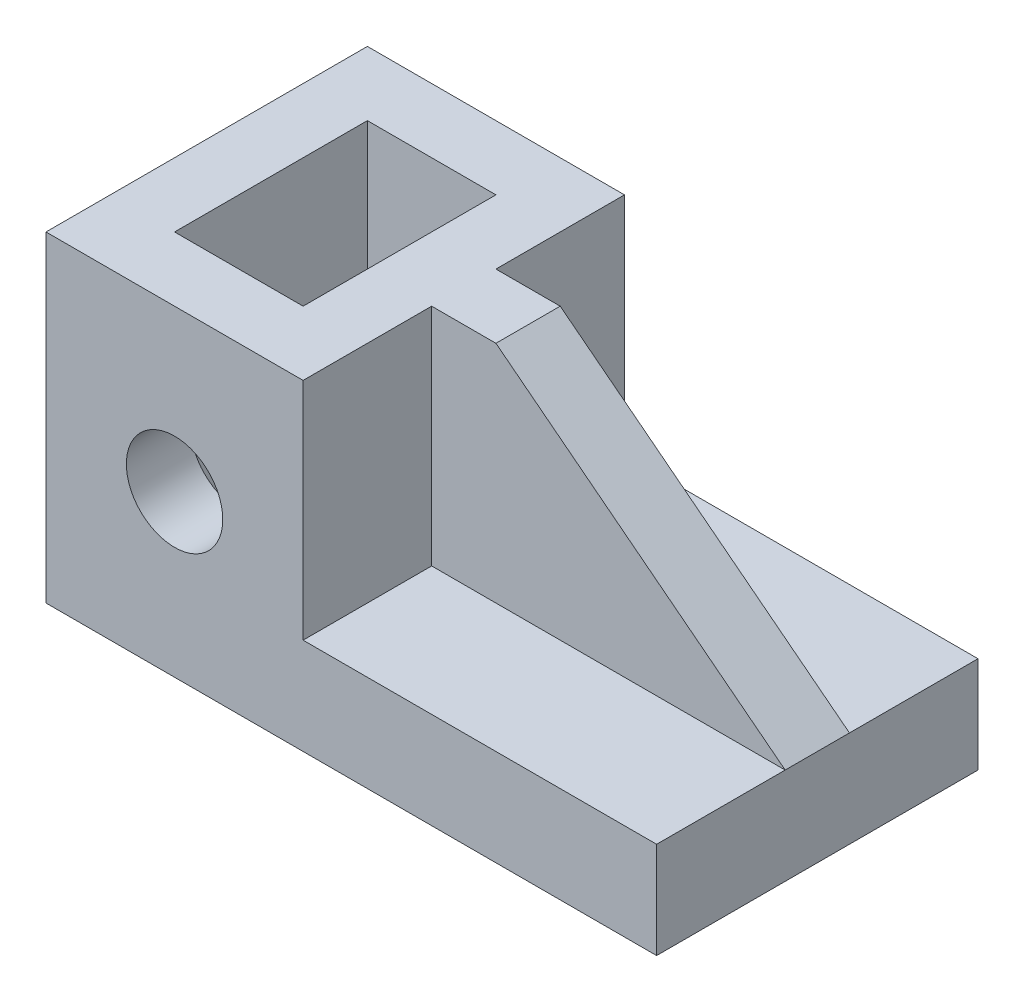
ISO-10303-21;
HEADER;
FILE_DESCRIPTION(('STEP AP214'),'2;1');
FILE_NAME('part.step','',(''),(''),'','','');
FILE_SCHEMA(('AUTOMOTIVE_DESIGN { 1 0 10303 214 1 1 1 1 }'));
ENDSEC;
DATA;
#1=APPLICATION_CONTEXT('core data for automotive mechanical design processes');
#2=APPLICATION_PROTOCOL_DEFINITION('international standard','automotive_design',2000,#1);
#3=PRODUCT_CONTEXT('',#1,'mechanical');
#4=PRODUCT('Part','Part','',(#3));
#5=PRODUCT_RELATED_PRODUCT_CATEGORY('part','',(#4));
#6=PRODUCT_DEFINITION_FORMATION('','',#4);
#7=PRODUCT_DEFINITION_CONTEXT('part definition',#1,'design');
#8=PRODUCT_DEFINITION('design','',#6,#7);
#9=PRODUCT_DEFINITION_SHAPE('','',#8);
#10=(LENGTH_UNIT() NAMED_UNIT(*) SI_UNIT(.MILLI.,.METRE.));
#11=(NAMED_UNIT(*) PLANE_ANGLE_UNIT() SI_UNIT($,.RADIAN.));
#12=(NAMED_UNIT(*) SI_UNIT($,.STERADIAN.) SOLID_ANGLE_UNIT());
#13=UNCERTAINTY_MEASURE_WITH_UNIT(LENGTH_MEASURE(1.E-05),#10,'distance_accuracy_value','');
#14=(GEOMETRIC_REPRESENTATION_CONTEXT(3) GLOBAL_UNCERTAINTY_ASSIGNED_CONTEXT((#13)) GLOBAL_UNIT_ASSIGNED_CONTEXT((#10,
#11,#12)) REPRESENTATION_CONTEXT('',''));
#15=CARTESIAN_POINT('',(0.,0.,0.));
#16=DIRECTION('',(0.,0.,1.));
#17=DIRECTION('',(1.,0.,0.));
#18=AXIS2_PLACEMENT_3D('',#15,#16,#17);
#19=CARTESIAN_POINT('',(40.,15.,50.));
#20=DIRECTION('',(0.,-1.,0.));
#21=DIRECTION('',(0.,0.,-1.));
#22=AXIS2_PLACEMENT_3D('',#19,#20,#21);
#23=PLANE('',#22);
#24=DIRECTION('',(-1.,0.,0.));
#25=VECTOR('',#24,1.);
#26=CARTESIAN_POINT('',(50.,15.,20.));
#27=LINE('',#26,#25);
#28=CARTESIAN_POINT('',(95.,15.,20.));
#29=VERTEX_POINT('',#28);
#30=CARTESIAN_POINT('',(40.,15.,20.));
#31=VERTEX_POINT('',#30);
#32=EDGE_CURVE('E189',#29,#31,#27,.T.);
#33=ORIENTED_EDGE('',*,*,#32,.F.);
#34=DIRECTION('',(0.,0.,-1.));
#35=VECTOR('',#34,1.);
#36=CARTESIAN_POINT('',(95.,15.,50.));
#37=LINE('',#36,#35);
#38=CARTESIAN_POINT('',(95.,15.,0.));
#39=VERTEX_POINT('',#38);
#40=EDGE_CURVE('E254',#29,#39,#37,.T.);
#41=ORIENTED_EDGE('',*,*,#40,.T.);
#42=DIRECTION('',(-1.,0.,0.));
#43=VECTOR('',#42,1.);
#44=CARTESIAN_POINT('',(40.,15.,0.));
#45=LINE('',#44,#43);
#46=CARTESIAN_POINT('',(40.,15.,0.));
#47=VERTEX_POINT('',#46);
#48=EDGE_CURVE('E236',#39,#47,#45,.T.);
#49=ORIENTED_EDGE('',*,*,#48,.T.);
#50=DIRECTION('',(0.,0.,-1.));
#51=VECTOR('',#50,1.);
#52=CARTESIAN_POINT('',(40.,15.,50.));
#53=LINE('',#52,#51);
#54=EDGE_CURVE('E253',#31,#47,#53,.T.);
#55=ORIENTED_EDGE('',*,*,#54,.F.);
#56=EDGE_LOOP('',(#33,#41,#49,#55));
#57=FACE_BOUND('',#56,.T.);
#58=ADVANCED_FACE('F39',(#57),#23,.F.);
#59=CARTESIAN_POINT('',(40.,50.,50.));
#60=DIRECTION('',(-1.,0.,0.));
#61=DIRECTION('',(0.,0.,1.));
#62=AXIS2_PLACEMENT_3D('',#59,#60,#61);
#63=PLANE('',#62);
#64=DIRECTION('',(0.,0.,-1.));
#65=VECTOR('',#64,1.);
#66=CARTESIAN_POINT('',(40.,50.,50.));
#67=LINE('',#66,#65);
#68=CARTESIAN_POINT('',(40.,50.,20.));
#69=VERTEX_POINT('',#68);
#70=CARTESIAN_POINT('',(40.,50.,0.));
#71=VERTEX_POINT('',#70);
#72=EDGE_CURVE('E250',#69,#71,#67,.T.);
#73=ORIENTED_EDGE('',*,*,#72,.F.);
#74=DIRECTION('',(0.,1.,0.));
#75=VECTOR('',#74,1.);
#76=CARTESIAN_POINT('',(40.,15.,20.));
#77=LINE('',#76,#75);
#78=EDGE_CURVE('E200',#31,#69,#77,.T.);
#79=ORIENTED_EDGE('',*,*,#78,.F.);
#80=ORIENTED_EDGE('',*,*,#54,.T.);
#81=DIRECTION('',(0.,1.,0.));
#82=VECTOR('',#81,1.);
#83=CARTESIAN_POINT('',(40.,50.,0.));
#84=LINE('',#83,#82);
#85=EDGE_CURVE('E242',#47,#71,#84,.T.);
#86=ORIENTED_EDGE('',*,*,#85,.T.);
#87=EDGE_LOOP('',(#73,#79,#80,#86));
#88=FACE_BOUND('',#87,.T.);
#89=ADVANCED_FACE('F297',(#88),#63,.F.);
#90=CARTESIAN_POINT('',(0.,0.,50.));
#91=DIRECTION('',(1.,0.,0.));
#92=DIRECTION('',(0.,0.,-1.));
#93=AXIS2_PLACEMENT_3D('',#90,#91,#92);
#94=PLANE('',#93);
#95=DIRECTION('',(0.,0.,-1.));
#96=VECTOR('',#95,1.);
#97=CARTESIAN_POINT('',(0.,50.,50.));
#98=LINE('',#97,#96);
#99=CARTESIAN_POINT('',(0.,50.,50.));
#100=VERTEX_POINT('',#99);
#101=CARTESIAN_POINT('',(0.,50.,0.));
#102=VERTEX_POINT('',#101);
#103=EDGE_CURVE('E229',#100,#102,#98,.T.);
#104=ORIENTED_EDGE('',*,*,#103,.T.);
#105=DIRECTION('',(0.,-1.,0.));
#106=VECTOR('',#105,1.);
#107=CARTESIAN_POINT('',(0.,0.,0.));
#108=LINE('',#107,#106);
#109=CARTESIAN_POINT('',(0.,0.,0.));
#110=VERTEX_POINT('',#109);
#111=EDGE_CURVE('E212',#102,#110,#108,.T.);
#112=ORIENTED_EDGE('',*,*,#111,.T.);
#113=DIRECTION('',(0.,0.,-1.));
#114=VECTOR('',#113,1.);
#115=CARTESIAN_POINT('',(0.,0.,50.));
#116=LINE('',#115,#114);
#117=CARTESIAN_POINT('',(0.,0.,50.));
#118=VERTEX_POINT('',#117);
#119=EDGE_CURVE('E11',#118,#110,#116,.T.);
#120=ORIENTED_EDGE('',*,*,#119,.F.);
#121=DIRECTION('',(0.,-1.,0.));
#122=VECTOR('',#121,1.);
#123=CARTESIAN_POINT('',(0.,0.,50.));
#124=LINE('',#123,#122);
#125=EDGE_CURVE('E214',#100,#118,#124,.T.);
#126=ORIENTED_EDGE('',*,*,#125,.F.);
#127=EDGE_LOOP('',(#104,#112,#120,#126));
#128=FACE_BOUND('',#127,.T.);
#129=ADVANCED_FACE('F41',(#128),#94,.F.);
#130=CARTESIAN_POINT('',(0.,0.,50.));
#131=DIRECTION('',(0.,1.,0.));
#132=DIRECTION('',(0.,0.,1.));
#133=AXIS2_PLACEMENT_3D('',#130,#131,#132);
#134=PLANE('',#133);
#135=DIRECTION('',(1.,0.,0.));
#136=VECTOR('',#135,1.);
#137=CARTESIAN_POINT('',(10.,0.,40.));
#138=LINE('',#137,#136);
#139=CARTESIAN_POINT('',(10.,0.,40.));
#140=VERTEX_POINT('',#139);
#141=CARTESIAN_POINT('',(30.,0.,40.));
#142=VERTEX_POINT('',#141);
#143=EDGE_CURVE('E150',#140,#142,#138,.T.);
#144=ORIENTED_EDGE('',*,*,#143,.T.);
#145=DIRECTION('',(0.,0.,-1.));
#146=VECTOR('',#145,1.);
#147=CARTESIAN_POINT('',(30.,0.,10.));
#148=LINE('',#147,#146);
#149=CARTESIAN_POINT('',(30.,0.,10.));
#150=VERTEX_POINT('',#149);
#151=EDGE_CURVE('E143',#142,#150,#148,.T.);
#152=ORIENTED_EDGE('',*,*,#151,.T.);
#153=DIRECTION('',(-1.,0.,0.));
#154=VECTOR('',#153,1.);
#155=CARTESIAN_POINT('',(10.,0.,10.));
#156=LINE('',#155,#154);
#157=CARTESIAN_POINT('',(10.,0.,10.));
#158=VERTEX_POINT('',#157);
#159=EDGE_CURVE('E147',#150,#158,#156,.T.);
#160=ORIENTED_EDGE('',*,*,#159,.T.);
#161=DIRECTION('',(0.,0.,1.));
#162=VECTOR('',#161,1.);
#163=CARTESIAN_POINT('',(10.,0.,10.));
#164=LINE('',#163,#162);
#165=EDGE_CURVE('E53',#158,#140,#164,.T.);
#166=ORIENTED_EDGE('',*,*,#165,.T.);
#167=EDGE_LOOP('',(#144,#152,#160,#166));
#168=FACE_BOUND('',#167,.T.);
#169=ORIENTED_EDGE('',*,*,#119,.T.);
#170=DIRECTION('',(1.,0.,0.));
#171=VECTOR('',#170,1.);
#172=CARTESIAN_POINT('',(0.,0.,0.));
#173=LINE('',#172,#171);
#174=CARTESIAN_POINT('',(95.,0.,0.));
#175=VERTEX_POINT('',#174);
#176=EDGE_CURVE('E235',#110,#175,#173,.T.);
#177=ORIENTED_EDGE('',*,*,#176,.T.);
#178=DIRECTION('',(0.,0.,-1.));
#179=VECTOR('',#178,1.);
#180=CARTESIAN_POINT('',(95.,0.,50.));
#181=LINE('',#180,#179);
#182=CARTESIAN_POINT('',(95.,0.,50.));
#183=VERTEX_POINT('',#182);
#184=EDGE_CURVE('E50',#183,#175,#181,.T.);
#185=ORIENTED_EDGE('',*,*,#184,.F.);
#186=DIRECTION('',(1.,0.,0.));
#187=VECTOR('',#186,1.);
#188=CARTESIAN_POINT('',(0.,0.,50.));
#189=LINE('',#188,#187);
#190=EDGE_CURVE('E217',#118,#183,#189,.T.);
#191=ORIENTED_EDGE('',*,*,#190,.F.);
#192=EDGE_LOOP('',(#169,#177,#185,#191));
#193=FACE_BOUND('',#192,.T.);
#194=ADVANCED_FACE('F152',(#168,#193),#134,.F.);
#195=CARTESIAN_POINT('',(95.,0.,50.));
#196=DIRECTION('',(-1.,0.,0.));
#197=DIRECTION('',(0.,0.,1.));
#198=AXIS2_PLACEMENT_3D('',#195,#196,#197);
#199=PLANE('',#198);
#200=ORIENTED_EDGE('',*,*,#184,.T.);
#201=DIRECTION('',(0.,1.,0.));
#202=VECTOR('',#201,1.);
#203=CARTESIAN_POINT('',(95.,0.,0.));
#204=LINE('',#203,#202);
#205=EDGE_CURVE('E234',#175,#39,#204,.T.);
#206=ORIENTED_EDGE('',*,*,#205,.T.);
#207=ORIENTED_EDGE('',*,*,#40,.F.);
#208=DIRECTION('',(0.,0.,-1.));
#209=VECTOR('',#208,1.);
#210=CARTESIAN_POINT('',(95.,15.,50.));
#211=LINE('',#210,#209);
#212=CARTESIAN_POINT('',(95.,15.,30.));
#213=VERTEX_POINT('',#212);
#214=EDGE_CURVE('E177',#29,#213,#211,.F.);
#215=ORIENTED_EDGE('',*,*,#214,.T.);
#216=CARTESIAN_POINT('',(95.,15.,50.));
#217=VERTEX_POINT('',#216);
#218=EDGE_CURVE('E258',#217,#213,#37,.T.);
#219=ORIENTED_EDGE('',*,*,#218,.F.);
#220=DIRECTION('',(0.,1.,0.));
#221=VECTOR('',#220,1.);
#222=CARTESIAN_POINT('',(95.,0.,50.));
#223=LINE('',#222,#221);
#224=EDGE_CURVE('E222',#183,#217,#223,.T.);
#225=ORIENTED_EDGE('',*,*,#224,.F.);
#226=EDGE_LOOP('',(#200,#206,#207,#215,#219,#225));
#227=FACE_BOUND('',#226,.T.);
#228=ADVANCED_FACE('F261',(#227),#199,.F.);
#229=ORIENTED_EDGE('',*,*,#218,.T.);
#230=DIRECTION('',(1.,0.,0.));
#231=VECTOR('',#230,1.);
#232=CARTESIAN_POINT('',(50.,15.,30.));
#233=LINE('',#232,#231);
#234=CARTESIAN_POINT('',(40.,15.,30.));
#235=VERTEX_POINT('',#234);
#236=EDGE_CURVE('E190',#235,#213,#233,.T.);
#237=ORIENTED_EDGE('',*,*,#236,.F.);
#238=CARTESIAN_POINT('',(40.,15.,50.));
#239=VERTEX_POINT('',#238);
#240=EDGE_CURVE('E252',#239,#235,#53,.T.);
#241=ORIENTED_EDGE('',*,*,#240,.F.);
#242=DIRECTION('',(-1.,0.,0.));
#243=VECTOR('',#242,1.);
#244=CARTESIAN_POINT('',(40.,15.,50.));
#245=LINE('',#244,#243);
#246=EDGE_CURVE('E224',#217,#239,#245,.T.);
#247=ORIENTED_EDGE('',*,*,#246,.F.);
#248=EDGE_LOOP('',(#229,#237,#241,#247));
#249=FACE_BOUND('',#248,.T.);
#250=ADVANCED_FACE('F278',(#249),#23,.F.);
#251=ORIENTED_EDGE('',*,*,#240,.T.);
#252=DIRECTION('',(0.,1.,0.));
#253=VECTOR('',#252,1.);
#254=CARTESIAN_POINT('',(40.,15.,30.));
#255=LINE('',#254,#253);
#256=CARTESIAN_POINT('',(40.,50.,30.));
#257=VERTEX_POINT('',#256);
#258=EDGE_CURVE('E195',#235,#257,#255,.T.);
#259=ORIENTED_EDGE('',*,*,#258,.T.);
#260=CARTESIAN_POINT('',(40.,50.,50.));
#261=VERTEX_POINT('',#260);
#262=EDGE_CURVE('E248',#261,#257,#67,.T.);
#263=ORIENTED_EDGE('',*,*,#262,.F.);
#264=DIRECTION('',(0.,1.,0.));
#265=VECTOR('',#264,1.);
#266=CARTESIAN_POINT('',(40.,50.,50.));
#267=LINE('',#266,#265);
#268=EDGE_CURVE('E223',#239,#261,#267,.T.);
#269=ORIENTED_EDGE('',*,*,#268,.F.);
#270=EDGE_LOOP('',(#251,#259,#263,#269));
#271=FACE_BOUND('',#270,.T.);
#272=ADVANCED_FACE('F302',(#271),#63,.F.);
#273=CARTESIAN_POINT('',(0.,50.,50.));
#274=DIRECTION('',(0.,-1.,0.));
#275=DIRECTION('',(0.,0.,-1.));
#276=AXIS2_PLACEMENT_3D('',#273,#274,#275);
#277=PLANE('',#276);
#278=DIRECTION('',(-1.,0.,0.));
#279=VECTOR('',#278,1.);
#280=CARTESIAN_POINT('',(10.,50.,10.));
#281=LINE('',#280,#279);
#282=CARTESIAN_POINT('',(30.,50.,10.));
#283=VERTEX_POINT('',#282);
#284=CARTESIAN_POINT('',(10.,50.,10.));
#285=VERTEX_POINT('',#284);
#286=EDGE_CURVE('E167',#283,#285,#281,.T.);
#287=ORIENTED_EDGE('',*,*,#286,.F.);
#288=DIRECTION('',(0.,0.,-1.));
#289=VECTOR('',#288,1.);
#290=CARTESIAN_POINT('',(30.,50.,10.));
#291=LINE('',#290,#289);
#292=CARTESIAN_POINT('',(30.,50.,40.));
#293=VERTEX_POINT('',#292);
#294=EDGE_CURVE('E65',#293,#283,#291,.T.);
#295=ORIENTED_EDGE('',*,*,#294,.F.);
#296=DIRECTION('',(1.,0.,0.));
#297=VECTOR('',#296,1.);
#298=CARTESIAN_POINT('',(10.,50.,40.));
#299=LINE('',#298,#297);
#300=CARTESIAN_POINT('',(10.,50.,40.));
#301=VERTEX_POINT('',#300);
#302=EDGE_CURVE('E160',#301,#293,#299,.T.);
#303=ORIENTED_EDGE('',*,*,#302,.F.);
#304=DIRECTION('',(0.,0.,1.));
#305=VECTOR('',#304,1.);
#306=CARTESIAN_POINT('',(10.,50.,10.));
#307=LINE('',#306,#305);
#308=EDGE_CURVE('E159',#285,#301,#307,.T.);
#309=ORIENTED_EDGE('',*,*,#308,.F.);
#310=EDGE_LOOP('',(#287,#295,#303,#309));
#311=FACE_BOUND('',#310,.T.);
#312=ORIENTED_EDGE('',*,*,#262,.T.);
#313=DIRECTION('',(1.,0.,0.));
#314=VECTOR('',#313,1.);
#315=CARTESIAN_POINT('',(50.,50.,30.));
#316=LINE('',#315,#314);
#317=CARTESIAN_POINT('',(50.,50.,30.));
#318=VERTEX_POINT('',#317);
#319=EDGE_CURVE('E187',#257,#318,#316,.T.);
#320=ORIENTED_EDGE('',*,*,#319,.T.);
#321=DIRECTION('',(0.,0.,-1.));
#322=VECTOR('',#321,1.);
#323=CARTESIAN_POINT('',(50.,50.,20.));
#324=LINE('',#323,#322);
#325=CARTESIAN_POINT('',(50.,50.,20.));
#326=VERTEX_POINT('',#325);
#327=EDGE_CURVE('E194',#318,#326,#324,.T.);
#328=ORIENTED_EDGE('',*,*,#327,.T.);
#329=DIRECTION('',(-1.,0.,0.));
#330=VECTOR('',#329,1.);
#331=CARTESIAN_POINT('',(50.,50.,20.));
#332=LINE('',#331,#330);
#333=EDGE_CURVE('E186',#326,#69,#332,.T.);
#334=ORIENTED_EDGE('',*,*,#333,.T.);
#335=ORIENTED_EDGE('',*,*,#72,.T.);
#336=DIRECTION('',(-1.,0.,0.));
#337=VECTOR('',#336,1.);
#338=CARTESIAN_POINT('',(0.,50.,0.));
#339=LINE('',#338,#337);
#340=EDGE_CURVE('E218',#71,#102,#339,.T.);
#341=ORIENTED_EDGE('',*,*,#340,.T.);
#342=ORIENTED_EDGE('',*,*,#103,.F.);
#343=DIRECTION('',(-1.,0.,0.));
#344=VECTOR('',#343,1.);
#345=CARTESIAN_POINT('',(0.,50.,50.));
#346=LINE('',#345,#344);
#347=EDGE_CURVE('E230',#261,#100,#346,.T.);
#348=ORIENTED_EDGE('',*,*,#347,.F.);
#349=EDGE_LOOP('',(#312,#320,#328,#334,#335,#341,#342,#348));
#350=FACE_BOUND('',#349,.T.);
#351=ADVANCED_FACE('F292',(#311,#350),#277,.F.);
#352=CARTESIAN_POINT('',(0.,0.,50.));
#353=DIRECTION('',(0.,0.,-1.));
#354=DIRECTION('',(-1.,0.,0.));
#355=AXIS2_PLACEMENT_3D('',#352,#353,#354);
#356=PLANE('',#355);
#357=CARTESIAN_POINT('',(20.,25.,50.));
#358=DIRECTION('',(0.,0.,1.));
#359=DIRECTION('',(1.,0.,0.));
#360=AXIS2_PLACEMENT_3D('',#357,#358,#359);
#361=CIRCLE('',#360,7.5);
#362=CARTESIAN_POINT('',(27.5,25.,50.));
#363=VERTEX_POINT('',#362);
#364=EDGE_CURVE('E207',#363,#363,#361,.T.);
#365=ORIENTED_EDGE('',*,*,#364,.F.);
#366=EDGE_LOOP('',(#365));
#367=FACE_BOUND('',#366,.T.);
#368=ORIENTED_EDGE('',*,*,#125,.T.);
#369=ORIENTED_EDGE('',*,*,#190,.T.);
#370=ORIENTED_EDGE('',*,*,#224,.T.);
#371=ORIENTED_EDGE('',*,*,#246,.T.);
#372=ORIENTED_EDGE('',*,*,#268,.T.);
#373=ORIENTED_EDGE('',*,*,#347,.T.);
#374=EDGE_LOOP('',(#368,#369,#370,#371,#372,#373));
#375=FACE_BOUND('',#374,.T.);
#376=ADVANCED_FACE('F284',(#367,#375),#356,.F.);
#377=CARTESIAN_POINT('',(0.,0.,0.));
#378=DIRECTION('',(0.,0.,-1.));
#379=DIRECTION('',(-1.,0.,0.));
#380=AXIS2_PLACEMENT_3D('',#377,#378,#379);
#381=PLANE('',#380);
#382=CARTESIAN_POINT('',(20.,25.,0.));
#383=DIRECTION('',(0.,0.,-1.));
#384=DIRECTION('',(-1.,0.,0.));
#385=AXIS2_PLACEMENT_3D('',#382,#383,#384);
#386=CIRCLE('',#385,7.5);
#387=CARTESIAN_POINT('',(12.5,25.,0.));
#388=VERTEX_POINT('',#387);
#389=EDGE_CURVE('E205',#388,#388,#386,.T.);
#390=ORIENTED_EDGE('',*,*,#389,.F.);
#391=EDGE_LOOP('',(#390));
#392=FACE_BOUND('',#391,.T.);
#393=ORIENTED_EDGE('',*,*,#111,.F.);
#394=ORIENTED_EDGE('',*,*,#340,.F.);
#395=ORIENTED_EDGE('',*,*,#85,.F.);
#396=ORIENTED_EDGE('',*,*,#48,.F.);
#397=ORIENTED_EDGE('',*,*,#205,.F.);
#398=ORIENTED_EDGE('',*,*,#176,.F.);
#399=EDGE_LOOP('',(#393,#394,#395,#396,#397,#398));
#400=FACE_BOUND('',#399,.T.);
#401=ADVANCED_FACE('F269',(#392,#400),#381,.T.);
#402=CARTESIAN_POINT('',(20.,25.,40.));
#403=DIRECTION('',(0.,0.,1.));
#404=DIRECTION('',(1.,0.,0.));
#405=AXIS2_PLACEMENT_3D('',#402,#403,#404);
#406=CYLINDRICAL_SURFACE('',#405,7.5);
#407=CARTESIAN_POINT('',(20.,25.,40.));
#408=DIRECTION('',(0.,0.,1.));
#409=DIRECTION('',(1.,0.,0.));
#410=AXIS2_PLACEMENT_3D('',#407,#408,#409);
#411=CIRCLE('',#410,7.5);
#412=CARTESIAN_POINT('',(27.5,25.,40.));
#413=VERTEX_POINT('',#412);
#414=EDGE_CURVE('E181',#413,#413,#411,.T.);
#415=ORIENTED_EDGE('',*,*,#414,.F.);
#416=EDGE_LOOP('',(#415));
#417=FACE_BOUND('',#416,.T.);
#418=ORIENTED_EDGE('',*,*,#364,.T.);
#419=EDGE_LOOP('',(#418));
#420=FACE_BOUND('',#419,.T.);
#421=ADVANCED_FACE('F405',(#417,#420),#406,.F.);
#422=CARTESIAN_POINT('',(20.,25.,10.));
#423=DIRECTION('',(0.,0.,-1.));
#424=DIRECTION('',(-1.,0.,0.));
#425=AXIS2_PLACEMENT_3D('',#422,#423,#424);
#426=CYLINDRICAL_SURFACE('',#425,7.5);
#427=CARTESIAN_POINT('',(20.,25.,10.));
#428=DIRECTION('',(0.,0.,-1.));
#429=DIRECTION('',(-1.,0.,0.));
#430=AXIS2_PLACEMENT_3D('',#427,#428,#429);
#431=CIRCLE('',#430,7.5);
#432=CARTESIAN_POINT('',(12.5,25.,10.));
#433=VERTEX_POINT('',#432);
#434=EDGE_CURVE('E175',#433,#433,#431,.T.);
#435=ORIENTED_EDGE('',*,*,#434,.F.);
#436=EDGE_LOOP('',(#435));
#437=FACE_BOUND('',#436,.T.);
#438=ORIENTED_EDGE('',*,*,#389,.T.);
#439=EDGE_LOOP('',(#438));
#440=FACE_BOUND('',#439,.T.);
#441=ADVANCED_FACE('F342',(#437,#440),#426,.F.);
#442=CARTESIAN_POINT('',(50.,15.,20.));
#443=DIRECTION('',(0.,0.,-1.));
#444=DIRECTION('',(-1.,0.,0.));
#445=AXIS2_PLACEMENT_3D('',#442,#443,#444);
#446=PLANE('',#445);
#447=ORIENTED_EDGE('',*,*,#333,.F.);
#448=DIRECTION('',(0.789352217376326,-0.61394061351492,0.));
#449=VECTOR('',#448,1.);
#450=CARTESIAN_POINT('',(50.,50.,20.));
#451=LINE('',#450,#449);
#452=EDGE_CURVE('E179',#326,#29,#451,.T.);
#453=ORIENTED_EDGE('',*,*,#452,.T.);
#454=ORIENTED_EDGE('',*,*,#32,.T.);
#455=ORIENTED_EDGE('',*,*,#78,.T.);
#456=EDGE_LOOP('',(#447,#453,#454,#455));
#457=FACE_BOUND('',#456,.T.);
#458=ADVANCED_FACE('F298',(#457),#446,.T.);
#459=CARTESIAN_POINT('',(50.,15.,30.));
#460=DIRECTION('',(0.,0.,1.));
#461=DIRECTION('',(1.,0.,0.));
#462=AXIS2_PLACEMENT_3D('',#459,#460,#461);
#463=PLANE('',#462);
#464=ORIENTED_EDGE('',*,*,#319,.F.);
#465=ORIENTED_EDGE('',*,*,#258,.F.);
#466=ORIENTED_EDGE('',*,*,#236,.T.);
#467=DIRECTION('',(0.789352217376326,-0.61394061351492,0.));
#468=VECTOR('',#467,1.);
#469=CARTESIAN_POINT('',(50.,50.,30.));
#470=LINE('',#469,#468);
#471=EDGE_CURVE('E176',#318,#213,#470,.T.);
#472=ORIENTED_EDGE('',*,*,#471,.F.);
#473=EDGE_LOOP('',(#464,#465,#466,#472));
#474=FACE_BOUND('',#473,.T.);
#475=ADVANCED_FACE('F305',(#474),#463,.T.);
#476=CARTESIAN_POINT('',(50.,50.,25.));
#477=DIRECTION('',(-0.61394061351492,-0.789352217376326,0.));
#478=DIRECTION('',(0.789352217376326,-0.61394061351492,0.));
#479=AXIS2_PLACEMENT_3D('',#476,#477,#478);
#480=PLANE('',#479);
#481=ORIENTED_EDGE('',*,*,#214,.F.);
#482=ORIENTED_EDGE('',*,*,#452,.F.);
#483=ORIENTED_EDGE('',*,*,#327,.F.);
#484=ORIENTED_EDGE('',*,*,#471,.T.);
#485=EDGE_LOOP('',(#481,#482,#483,#484));
#486=FACE_BOUND('',#485,.T.);
#487=ADVANCED_FACE('F296',(#486),#480,.F.);
#488=CARTESIAN_POINT('',(30.,0.,10.));
#489=DIRECTION('',(1.,0.,0.));
#490=DIRECTION('',(0.,0.,-1.));
#491=AXIS2_PLACEMENT_3D('',#488,#489,#490);
#492=PLANE('',#491);
#493=ORIENTED_EDGE('',*,*,#294,.T.);
#494=DIRECTION('',(0.,1.,0.));
#495=VECTOR('',#494,1.);
#496=CARTESIAN_POINT('',(30.,0.,10.));
#497=LINE('',#496,#495);
#498=EDGE_CURVE('E140',#150,#283,#497,.T.);
#499=ORIENTED_EDGE('',*,*,#498,.F.);
#500=ORIENTED_EDGE('',*,*,#151,.F.);
#501=DIRECTION('',(0.,1.,0.));
#502=VECTOR('',#501,1.);
#503=CARTESIAN_POINT('',(30.,0.,40.));
#504=LINE('',#503,#502);
#505=EDGE_CURVE('E168',#142,#293,#504,.T.);
#506=ORIENTED_EDGE('',*,*,#505,.T.);
#507=EDGE_LOOP('',(#493,#499,#500,#506));
#508=FACE_BOUND('',#507,.T.);
#509=ADVANCED_FACE('F137',(#508),#492,.F.);
#510=CARTESIAN_POINT('',(10.,0.,40.));
#511=DIRECTION('',(0.,0.,1.));
#512=DIRECTION('',(1.,0.,0.));
#513=AXIS2_PLACEMENT_3D('',#510,#511,#512);
#514=PLANE('',#513);
#515=ORIENTED_EDGE('',*,*,#414,.T.);
#516=EDGE_LOOP('',(#515));
#517=FACE_BOUND('',#516,.T.);
#518=ORIENTED_EDGE('',*,*,#302,.T.);
#519=ORIENTED_EDGE('',*,*,#505,.F.);
#520=ORIENTED_EDGE('',*,*,#143,.F.);
#521=DIRECTION('',(0.,1.,0.));
#522=VECTOR('',#521,1.);
#523=CARTESIAN_POINT('',(10.,0.,40.));
#524=LINE('',#523,#522);
#525=EDGE_CURVE('E173',#140,#301,#524,.T.);
#526=ORIENTED_EDGE('',*,*,#525,.T.);
#527=EDGE_LOOP('',(#518,#519,#520,#526));
#528=FACE_BOUND('',#527,.T.);
#529=ADVANCED_FACE('F369',(#517,#528),#514,.F.);
#530=CARTESIAN_POINT('',(10.,0.,10.));
#531=DIRECTION('',(-1.,0.,0.));
#532=DIRECTION('',(0.,0.,1.));
#533=AXIS2_PLACEMENT_3D('',#530,#531,#532);
#534=PLANE('',#533);
#535=ORIENTED_EDGE('',*,*,#308,.T.);
#536=ORIENTED_EDGE('',*,*,#525,.F.);
#537=ORIENTED_EDGE('',*,*,#165,.F.);
#538=DIRECTION('',(0.,1.,0.));
#539=VECTOR('',#538,1.);
#540=CARTESIAN_POINT('',(10.,0.,10.));
#541=LINE('',#540,#539);
#542=EDGE_CURVE('E148',#158,#285,#541,.T.);
#543=ORIENTED_EDGE('',*,*,#542,.T.);
#544=EDGE_LOOP('',(#535,#536,#537,#543));
#545=FACE_BOUND('',#544,.T.);
#546=ADVANCED_FACE('F378',(#545),#534,.F.);
#547=CARTESIAN_POINT('',(10.,0.,10.));
#548=DIRECTION('',(0.,0.,-1.));
#549=DIRECTION('',(-1.,0.,0.));
#550=AXIS2_PLACEMENT_3D('',#547,#548,#549);
#551=PLANE('',#550);
#552=ORIENTED_EDGE('',*,*,#434,.T.);
#553=EDGE_LOOP('',(#552));
#554=FACE_BOUND('',#553,.T.);
#555=ORIENTED_EDGE('',*,*,#286,.T.);
#556=ORIENTED_EDGE('',*,*,#542,.F.);
#557=ORIENTED_EDGE('',*,*,#159,.F.);
#558=ORIENTED_EDGE('',*,*,#498,.T.);
#559=EDGE_LOOP('',(#555,#556,#557,#558));
#560=FACE_BOUND('',#559,.T.);
#561=ADVANCED_FACE('F151',(#554,#560),#551,.F.);
#562=CLOSED_SHELL('',(#58,#89,#129,#194,#228,#250,#272,#351,#376,#401,#421,#441,#458,#475,#487,
#509,#529,#546,#561));
#563=MANIFOLD_SOLID_BREP('B2',#562);
#564=ADVANCED_BREP_SHAPE_REPRESENTATION('',(#18,#563),#14);
#565=SHAPE_DEFINITION_REPRESENTATION(#9,#564);
ENDSEC;
END-ISO-10303-21;
